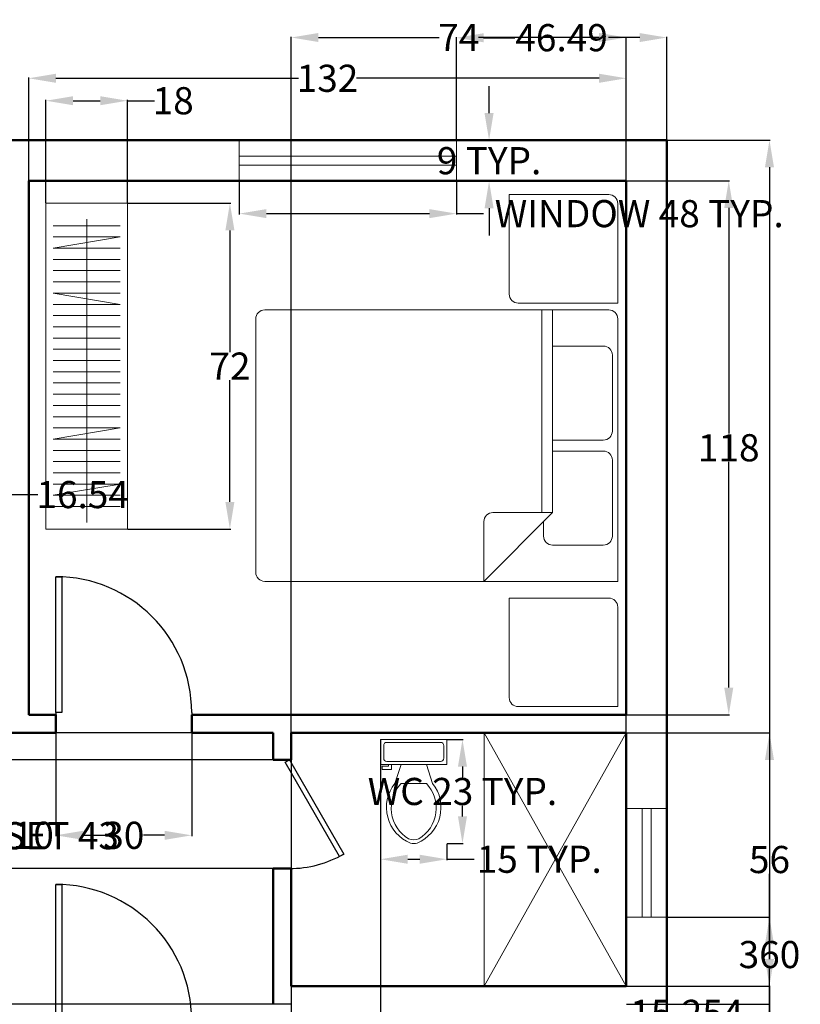
# Model space of a CAD drawing. Units: inches. Extents: x -8 to 300, y -428 to 46.
# Tile 4 of 4: x 122 to 294, y -172 to 46. Entities that reach past the tile are written whole.
import ezdxf

# ---------------------------------------------------------------- set-up
doc = ezdxf.new("R2010")
doc.units = ezdxf.units.IN
doc.header["$MEASUREMENT"] = 0
for name, color, linetype, lineweight in [('A-ANNO-DIMS', 2, 'Continuous', 18), ('A-DOOR', 3, 'Continuous', 25), ('A-FLOR-CASE', 9, 'Continuous', 18), ('A-FLOR-FIXT', 9, 'Continuous', 18), ('A-FURN', 8, 'Continuous', 18), ('A-GLAZ', 4, 'Continuous', 18), ('A-WALL', 7, 'Continuous', 50)]:
    doc.layers.add(name, color=color, linetype=linetype, lineweight=lineweight)
doc.styles.get("Standard").update_dxf_attribs({"font": 'arial.ttf'})
doc.dimstyles.get("Standard").update_dxf_attribs({"dimtxt": 6, "dimasz": 6, "dimexe": 0.18, "dimexo": 0.0625, "dimgap": 0.09, "dimtad": 0, "dimtih": 1, "dimtoh": 1, "dimdec": 0, "dimzin": 0, "dimdsep": 46, "dimlunit": 4, "dimtxsty": 'Standard', "dimcen": 0.09, "dimadec": 0, "dimazin": 0, "dimtfac": 1, "dimtdec": 0, "dimtofl": 0, "dimtmove": 0, "dimatfit": 3, "dimfxl": 1, "dimtolj": 1, "dimtzin": 0, "dimarcsym": 0})

# ---------------------------------------------------------------- blocks, each defined once
blk = doc.blocks.new('*U2')
for p, q in [((0, 0), (0, -6)), ((40, 0), (40, -6))]:
    blk.add_line(p, q)
blk.add_lwpolyline([(0, 0), (0, 40), (1.75, 40), (1.75, 0)], close=True)
blk.add_arc((0, 0), 40, 0, 90)
blk = doc.blocks.new('*U11')
for p, q in [((0, 0), (0, -6)), ((40, 0), (40, -6))]:
    blk.add_line(p, q)
blk.add_lwpolyline([(0, 0), (34.64, 20), (35.52, 18.48), (0.87, -1.52)], close=True)
blk.add_arc((0, 0), 40, 0, 30)
blk = doc.blocks.new('Toilet - top')
for p, q in [((9.5, -6), (9.5, -2)), ((-10, -8.5), (-8, -8.5)), ((-10, -9.5), (-10, -8.5)), ((-8, -8.5), (-8, -8)), ((-7, -8), (-7, -9.5)), ((-4, -8), (-6, -14)), ((4, -8), (6, -14)), ((-7, -9.5), (-10, -9.5)), ((4, -14), (-4, -14))]:
    blk.add_line(p, q)
blk.add_lwpolyline([(10.5, -8), (10.5, 0), (-10.5, 0), (-10.5, -8)], close=True)
for points in [[(-9.5, -2), (-9.5, -6)], [(8.5, -1), (-8.5, -1)], [(-8.5, -7), (8.5, -7)]]:
    blk.add_lwpolyline(points)
for centre, radius, start, end in [((-8.62, -1.88), 0.884, 81.8699, 188.1301), ((8.62, -1.88), 0.884, 351.8699, 98.1301), ((-8.62, -6.12), 0.884, 171.8699, 278.1301), ((8.62, -6.12), 0.884, 261.8699, 8.1301), ((3.52, -21.58), 12.17, 141.4691, 247.9714), ((4.2, -21.82), 11.33, 136.3677, 238.9468), ((-3.52, -21.58), 12.17, 292.0284, 38.5307), ((-4.2, -21.82), 11.33, 301.053, 43.6321), ((0, -27.88), 4, 245.7318, 294.2682), ((0, -29), 4, 254.8605, 285.1395)]:
    blk.add_arc(centre, radius, start, end)
blk = doc.blocks.new('Bed - Queen')
for p, q in [((2, 0), (60, 0)), ((60, 0), (60, -78)), ((0, -78), (0, -2)), ((10, -1.2), (26.8, -1.2)), ((33.2, -1.2), (50, -1.2)), ((8, -14.4), (8, -3.2)), ((28.8, -3.2), (28.8, -14.4)), ((31.2, -14.4), (31.2, -3.2)), ((52, -3.2), (52, -14.4)), ((0, -14.4), (44.8, -14.4)), ((60, -29.6), (44.8, -14.4)), ((44.8, -14.4), (44.8, -27.6)), ((44.8, -16.8), (0, -16.8)), ((50, -16.4), (46.8, -16.4)), ((46.8, -29.6), (60, -29.6)), ((58, -80), (2, -80))]:
    blk.add_line(p, q)
for points in [[(-1.48, 0), (-23.48, 0, 0.414214), (-25.48, -2), (-25.48, -24), (-3.48, -24, 0.414214), (-1.48, -22)], [(65.69, 0), (87.69, 0), (87.69, -22, -0.414214), (85.69, -24), (63.69, -24), (63.69, -2, -0.414214)]]:
    blk.add_lwpolyline(points, format="xyb", close=True)
for centre, start, end in [((2, -2), 90, 180), ((10, -3.2), 90, 180), ((26.8, -3.2), 0, 90), ((33.2, -3.2), 90, 180), ((50, -3.2), 0, 90), ((50, -14.4), 270, 0), ((46.8, -27.6), 180, 270), ((2, -78), 180, 270), ((58, -78), 270, 0)]:
    blk.add_arc(centre, 2, start, end)
blk = doc.blocks.new('WIN-48IN')
for p, q in [((0, 0), (0, 9)), ((48, 9), (48, 0)), ((0, 5.5), (48, 5.5)), ((0, 3.5), (48, 3.5))]:
    blk.add_line(p, q)
blk = doc.blocks.new('WIN-24IN')
for p, q in [((0, 24), (9, 24)), ((3.5, 24), (3.5, 0)), ((5.5, 24), (5.5, 0)), ((9, 0), (0, 0))]:
    blk.add_line(p, q)
blk = doc.blocks.new('*D15')
at = {"layer": 'A-ANNO-DIMS', "color": 0, "lineweight": -2, "transparency": 16777216}
for p, q in [((216.31, -113.16), (219.88, -113.16)), ((219.7, -119.16), (219.7, -121.48)), ((219.7, -130.19), (219.7, -127.87)), ((216.31, -136.19), (219.88, -136.19))]:
    blk.add_line(p, q, dxfattribs=at)
at = {"layer": 'A-ANNO-DIMS', "color": 0, "transparency": 16777216}
for points in [[(218.7, -119.16), (220.7, -119.16), (219.7, -113.16)], [(218.7, -130.19), (220.7, -130.19), (219.7, -136.19)]]:
    blk.add_solid(points, dxfattribs=at)
at = {"layer": 'Defpoints', "color": 0, "transparency": 16777216}
for p in [(216.25, -113.16), (219.7, -113.16), (216.25, -136.19)]:
    blk.add_point(p, dxfattribs=at)
at = {"layer": 'A-ANNO-DIMS', "color": 0, "transparency": 16777216, "insert": (219.7, -124.67), "char_height": 6, "attachment_point": 5}
blk.add_mtext('\\A1;WC 23 TYP.', dxfattribs=at)
blk = doc.blocks.new('*D16')
at = {"layer": 'A-ANNO-DIMS', "color": 0, "lineweight": -2, "transparency": 16777216}
for p, q in [((201.61, -136.25), (201.61, -139.83)), ((216.25, -136.25), (216.25, -139.83)), ((207.61, -139.65), (210.25, -139.65)), ((216.25, -139.65), (222.25, -139.65))]:
    blk.add_line(p, q, dxfattribs=at)
at = {"layer": 'A-ANNO-DIMS', "color": 0, "transparency": 16777216}
for points in [[(207.61, -138.65), (207.61, -140.65), (201.61, -139.65)], [(210.25, -138.65), (210.25, -140.65), (216.25, -139.65)]]:
    blk.add_solid(points, dxfattribs=at)
at = {"layer": 'Defpoints', "color": 0, "transparency": 16777216}
for p in [(201.61, -136.19), (216.25, -136.19), (216.25, -139.65)]:
    blk.add_point(p, dxfattribs=at)
at = {"layer": 'A-ANNO-DIMS', "color": 0, "transparency": 16777216, "insert": (236.66, -139.65), "char_height": 6, "attachment_point": 5}
blk.add_mtext('\\A1;15 TYP.', dxfattribs=at)
blk = doc.blocks.new('*D19')
at = {"layer": 'A-ANNO-DIMS', "color": 0, "lineweight": -2, "transparency": 16777216}
for p, q in [((170.38, 10.17), (170.38, 2.85)), ((218.38, 10.17), (218.38, 2.85)), ((176.38, 3.03), (212.38, 3.03)), ((218.38, 3.03), (224.38, 3.03))]:
    blk.add_line(p, q, dxfattribs=at)
at = {"layer": 'A-ANNO-DIMS', "color": 0, "transparency": 16777216}
for points in [[(176.38, 4.03), (176.38, 2.03), (170.38, 3.03)], [(212.38, 4.03), (212.38, 2.03), (218.38, 3.03)]]:
    blk.add_solid(points, dxfattribs=at)
at = {"layer": 'Defpoints', "color": 0, "transparency": 16777216}
for p in [(170.38, 10.23), (218.38, 10.23), (218.38, 3.03)]:
    blk.add_point(p, dxfattribs=at)
at = {"layer": 'A-ANNO-DIMS', "color": 0, "transparency": 16777216, "insert": (258.75, 3.03), "char_height": 6, "attachment_point": 5}
blk.add_mtext('\\A1;WINDOW 48 TYP.', dxfattribs=at)
blk = doc.blocks.new('*D20')
at = {"layer": 'A-ANNO-DIMS', "color": 0, "lineweight": -2, "transparency": 16777216}
for p, q in [((225.58, 25.23), (225.58, 31.23)), ((218.45, 19.23), (225.76, 19.23)), ((218.45, 10.23), (225.76, 10.23)), ((225.58, 4.23), (225.58, -1.77))]:
    blk.add_line(p, q, dxfattribs=at)
at = {"layer": 'A-ANNO-DIMS', "color": 0, "transparency": 16777216}
for points in [[(224.58, 25.23), (226.58, 25.23), (225.58, 19.23)], [(224.58, 4.23), (226.58, 4.23), (225.58, 10.23)]]:
    blk.add_solid(points, dxfattribs=at)
at = {"layer": 'Defpoints', "color": 0, "transparency": 16777216}
for p in [(218.38, 19.23), (225.58, 19.23), (218.38, 10.23)]:
    blk.add_point(p, dxfattribs=at)
at = {"layer": 'A-ANNO-DIMS', "color": 0, "transparency": 16777216, "insert": (225.58, 14.73), "char_height": 6, "attachment_point": 5}
blk.add_mtext('\\A1;9 TYP.', dxfattribs=at)
blk = doc.blocks.new('*D23')
at = {"layer": 'A-ANNO-DIMS', "color": 0, "lineweight": -2, "transparency": 16777216}
for p, q in [((37.97, -128.08), (37.97, -134.62)), ((80.78, -128.08), (80.78, -134.62)), ((43.97, -134.44), (74.78, -134.44)), ((80.78, -134.44), (86.78, -134.44))]:
    blk.add_line(p, q, dxfattribs=at)
at = {"layer": 'A-ANNO-DIMS', "color": 0, "transparency": 16777216}
for points in [[(43.97, -133.44), (43.97, -135.44), (37.97, -134.44)], [(74.78, -133.44), (74.78, -135.44), (80.78, -134.44)]]:
    blk.add_solid(points, dxfattribs=at)
at = {"layer": 'Defpoints', "color": 0, "transparency": 16777216}
for p in [(37.97, -128.02), (80.78, -128.02), (80.78, -134.44)]:
    blk.add_point(p, dxfattribs=at)
at = {"layer": 'A-ANNO-DIMS', "color": 0, "transparency": 16777216, "insert": (116.16, -134.44), "char_height": 6, "attachment_point": 5}
blk.add_mtext('\\A1;DINING SET 43', dxfattribs=at)
blk = doc.blocks.new('*D33')
at = {"layer": 'A-ANNO-DIMS', "color": 0, "lineweight": -2, "transparency": 16777216}
for p, q in [((264.94, 19.29), (287.71, 19.29)), ((287.53, 13.29), (287.53, -157.55)), ((287.53, -334.71), (287.53, -163.86)), ((264.94, -340.71), (287.71, -340.71))]:
    blk.add_line(p, q, dxfattribs=at)
at = {"layer": 'A-ANNO-DIMS', "color": 0, "transparency": 16777216}
for points in [[(286.53, 13.29), (288.53, 13.29), (287.53, 19.29)], [(286.53, -334.71), (288.53, -334.71), (287.53, -340.71)]]:
    blk.add_solid(points, dxfattribs=at)
at = {"layer": 'Defpoints', "color": 0, "transparency": 16777216}
for p in [(264.88, 19.29), (264.88, -340.71), (287.53, -340.71)]:
    blk.add_point(p, dxfattribs=at)
at = {"layer": 'A-ANNO-DIMS', "color": 0, "transparency": 16777216, "insert": (287.53, -160.71), "char_height": 6, "attachment_point": 5}
blk.add_mtext('\\A1;360', dxfattribs=at)
blk = doc.blocks.new('*D37')
at = {"layer": 'A-ANNO-DIMS', "color": 0, "lineweight": -2, "transparency": 16777216}
for p, q in [((123.88, 10.36), (123.88, 33.12)), ((129.88, 32.94), (183.47, 32.94)), ((249.88, 32.94), (196.28, 32.94)), ((255.88, 10.36), (255.88, 33.12))]:
    blk.add_line(p, q, dxfattribs=at)
at = {"layer": 'A-ANNO-DIMS', "color": 0, "transparency": 16777216}
for points in [[(129.88, 33.94), (129.88, 31.94), (123.88, 32.94)], [(249.88, 33.94), (249.88, 31.94), (255.88, 32.94)]]:
    blk.add_solid(points, dxfattribs=at)
at = {"layer": 'Defpoints', "color": 0, "transparency": 16777216}
for p in [(255.88, 32.94), (123.88, 10.29), (255.88, 10.29)]:
    blk.add_point(p, dxfattribs=at)
at = {"layer": 'A-ANNO-DIMS', "color": 0, "transparency": 16777216, "insert": (189.88, 32.94), "char_height": 6, "attachment_point": 5}
blk.add_mtext('\\A1;132', dxfattribs=at)
blk = doc.blocks.new('*D39')
at = {"layer": 'A-ANNO-DIMS', "color": 0, "lineweight": -2, "transparency": 16777216}
for p, q in [((255.94, 10.29), (278.71, 10.29)), ((278.53, 4.29), (278.53, -45.55)), ((278.53, -101.71), (278.53, -51.86)), ((255.94, -107.71), (278.71, -107.71))]:
    blk.add_line(p, q, dxfattribs=at)
at = {"layer": 'A-ANNO-DIMS', "color": 0, "transparency": 16777216}
for points in [[(277.53, 4.29), (279.53, 4.29), (278.53, 10.29)], [(277.53, -101.71), (279.53, -101.71), (278.53, -107.71)]]:
    blk.add_solid(points, dxfattribs=at)
at = {"layer": 'Defpoints', "color": 0, "transparency": 16777216}
for p in [(255.88, 10.29), (255.88, -107.71), (278.53, -107.71)]:
    blk.add_point(p, dxfattribs=at)
at = {"layer": 'A-ANNO-DIMS', "color": 0, "transparency": 16777216, "insert": (278.53, -48.71), "char_height": 6, "attachment_point": 5}
blk.add_mtext('\\A1;118', dxfattribs=at)
blk = doc.blocks.new('*D44')
at = {"layer": 'A-ANNO-DIMS', "color": 0, "lineweight": -2, "transparency": 16777216}
for p, q in [((129.88, -111.77), (129.88, -134.54)), ((159.88, -111.77), (159.88, -134.54)), ((135.88, -134.36), (140.5, -134.36)), ((153.88, -134.36), (149.25, -134.36))]:
    blk.add_line(p, q, dxfattribs=at)
at = {"layer": 'A-ANNO-DIMS', "color": 0, "transparency": 16777216}
for points in [[(135.88, -133.36), (135.88, -135.36), (129.88, -134.36)], [(153.88, -133.36), (153.88, -135.36), (159.88, -134.36)]]:
    blk.add_solid(points, dxfattribs=at)
at = {"layer": 'Defpoints', "color": 0, "transparency": 16777216}
for p in [(129.88, -111.71), (159.88, -111.71), (129.88, -134.36)]:
    blk.add_point(p, dxfattribs=at)
at = {"layer": 'A-ANNO-DIMS', "color": 0, "transparency": 16777216, "insert": (144.88, -134.36), "char_height": 6, "attachment_point": 5}
blk.add_mtext('\\A1;30', dxfattribs=at)
blk = doc.blocks.new('*D45')
at = {"layer": 'A-ANNO-DIMS', "color": 0, "lineweight": -2, "transparency": 16777216}
for p, q in [((119.875934, -111.769234), (119.875934, -134.536734)), ((129.875934, -111.769234), (129.875934, -134.536734)), ((113.875934, -134.356734), (107.875934, -134.356734)), ((135.875934, -134.356734), (141.875934, -134.356734))]:
    blk.add_line(p, q, dxfattribs=at)
at = {"layer": 'A-ANNO-DIMS', "color": 0, "transparency": 16777216}
for points in [[(113.875934, -133.356734), (113.875934, -135.356734), (119.875934, -134.356734)], [(135.875934, -133.356734), (135.875934, -135.356734), (129.875934, -134.356734)]]:
    blk.add_solid(points, dxfattribs=at)
at = {"layer": 'Defpoints', "color": 0, "transparency": 16777216}
for p in [(119.875934, -111.706734), (129.875934, -111.706734), (119.875934, -134.356734)]:
    blk.add_point(p, dxfattribs=at)
at = {"layer": 'A-ANNO-DIMS', "color": 0, "transparency": 16777216, "insert": (124.875934, -134.356734), "char_height": 6, "attachment_point": 5}
blk.add_mtext('\\A1;10', dxfattribs=at)
blk = doc.blocks.new('*D47')
at = {"layer": 'A-ANNO-DIMS', "color": 0, "lineweight": -2, "transparency": 16777216}
for p, q in [((103.33, -81.64), (103.33, -58.88)), ((109.33, -59.06), (113.88, -59.06)), ((119.88, -81.64), (119.88, -58.88)), ((119.88, -59.06), (125.88, -59.06))]:
    blk.add_line(p, q, dxfattribs=at)
at = {"layer": 'A-ANNO-DIMS', "color": 0, "transparency": 16777216}
for points in [[(109.33, -58.06), (109.33, -60.06), (103.33, -59.06)], [(113.88, -58.06), (113.88, -60.06), (119.88, -59.06)]]:
    blk.add_solid(points, dxfattribs=at)
at = {"layer": 'Defpoints', "color": 0, "transparency": 16777216}
for p in [(119.88, -59.06), (103.33, -81.71), (119.88, -81.71)]:
    blk.add_point(p, dxfattribs=at)
at = {"layer": 'A-ANNO-DIMS', "color": 0, "transparency": 16777216, "insert": (135.79, -59.06), "char_height": 6, "attachment_point": 5}
blk.add_mtext('\\A1;16.54', dxfattribs=at)
blk = doc.blocks.new('*D49')
at = {"layer": 'A-ANNO-DIMS', "color": 0, "lineweight": -2, "transparency": 16777216}
for p, q in [((218.38, 19.29), (218.35, 42.06)), ((224.35, 41.89), (231.26, 41.9)), ((258.85, 41.94), (251.94, 41.93)), ((264.88, 19.36), (264.85, 42.12))]:
    blk.add_line(p, q, dxfattribs=at)
at = {"layer": 'A-ANNO-DIMS', "color": 0, "transparency": 16777216}
for points in [[(224.35, 42.89), (224.36, 40.89), (218.35, 41.88)], [(258.84, 42.94), (258.85, 40.94), (264.85, 41.94)]]:
    blk.add_solid(points, dxfattribs=at)
at = {"layer": 'Defpoints', "color": 0, "transparency": 16777216}
for p in [(264.85, 41.94), (218.38, 19.23), (264.88, 19.29)]:
    blk.add_point(p, dxfattribs=at)
at = {"layer": 'A-ANNO-DIMS', "color": 0, "transparency": 16777216, "insert": (241.6, 41.91), "char_height": 6, "attachment_point": 5}
blk.add_mtext('\\A1;46.49', dxfattribs=at)
blk = doc.blocks.new('*D52')
at = {"layer": 'A-ANNO-DIMS', "color": 0, "lineweight": -2, "transparency": 16777216}
for p, q in [((181.88, -111.64), (181.88, 42.13)), ((187.88, 41.95), (214.53, 41.95)), ((249.88, 41.95), (223.23, 41.95)), ((255.88, -111.64), (255.88, 42.13))]:
    blk.add_line(p, q, dxfattribs=at)
at = {"layer": 'A-ANNO-DIMS', "color": 0, "transparency": 16777216}
for points in [[(187.88, 42.95), (187.88, 40.95), (181.88, 41.95)], [(249.88, 42.95), (249.88, 40.95), (255.88, 41.95)]]:
    blk.add_solid(points, dxfattribs=at)
at = {"layer": 'Defpoints', "color": 0, "transparency": 16777216}
for p in [(255.88, 41.95), (181.88, -111.71), (255.88, -111.71)]:
    blk.add_point(p, dxfattribs=at)
at = {"layer": 'A-ANNO-DIMS', "color": 0, "transparency": 16777216, "insert": (218.88, 41.95), "char_height": 6, "attachment_point": 5}
blk.add_mtext('\\A1;74', dxfattribs=at)
blk = doc.blocks.new('*D53')
at = {"layer": 'A-ANNO-DIMS', "color": 0, "lineweight": -2, "transparency": 16777216}
for p, q in [((255.94, -111.71), (287.71, -111.71)), ((287.53, -117.71), (287.53, -136.55)), ((287.53, -161.71), (287.53, -142.86)), ((255.94, -167.71), (287.71, -167.71))]:
    blk.add_line(p, q, dxfattribs=at)
at = {"layer": 'A-ANNO-DIMS', "color": 0, "transparency": 16777216}
for points in [[(286.53, -117.71), (288.53, -117.71), (287.53, -111.71)], [(286.53, -161.71), (288.53, -161.71), (287.53, -167.71)]]:
    blk.add_solid(points, dxfattribs=at)
at = {"layer": 'Defpoints', "color": 0, "transparency": 16777216}
for p in [(255.88, -111.71), (255.88, -167.71), (287.53, -167.71)]:
    blk.add_point(p, dxfattribs=at)
at = {"layer": 'A-ANNO-DIMS', "color": 0, "transparency": 16777216, "insert": (287.53, -139.71), "char_height": 6, "attachment_point": 5}
blk.add_mtext('\\A1;56', dxfattribs=at)
blk = doc.blocks.new('*D55')
at = {"layer": 'A-ANNO-DIMS', "color": 0, "lineweight": -2, "transparency": 16777216}
for p, q in [((287.53, -161.71), (287.53, -155.71)), ((255.94, -167.71), (287.71, -167.71)), ((255.94, -171.71), (287.71, -171.71)), ((287.53, -177.71), (287.53, -183.71)), ((287.53, -183.71), (281.53, -183.71))]:
    blk.add_line(p, q, dxfattribs=at)
at = {"layer": 'A-ANNO-DIMS', "color": 0, "transparency": 16777216}
for points in [[(286.53, -161.71), (288.53, -161.71), (287.53, -167.71)], [(286.53, -177.71), (288.53, -177.71), (287.53, -171.71)]]:
    blk.add_solid(points, dxfattribs=at)
at = {"layer": 'Defpoints', "color": 0, "transparency": 16777216}
for p in [(255.88, -167.71), (255.88, -171.71), (287.53, -171.71)]:
    blk.add_point(p, dxfattribs=at)
at = {"layer": 'A-ANNO-DIMS', "color": 0, "transparency": 16777216, "insert": (279.36, -183.71), "char_height": 6, "attachment_point": 5}
blk.add_mtext('\\A1;4', dxfattribs=at)
blk = doc.blocks.new('*D56')
at = {"layer": 'A-ANNO-DIMS', "color": 0, "lineweight": -2, "transparency": 16777216}
for p, q in [((177.81, -117.71), (2.05, -117.71)), ((2.23, -123.71), (2.23, -126.6)), ((2.23, -135.71), (2.23, -132.81)), ((177.81, -141.71), (2.05, -141.71))]:
    blk.add_line(p, q, dxfattribs=at)
at = {"layer": 'A-ANNO-DIMS', "color": 0, "transparency": 16777216}
for points in [[(1.23, -123.71), (3.23, -123.71), (2.23, -117.71)], [(1.23, -135.71), (3.23, -135.71), (2.23, -141.71)]]:
    blk.add_solid(points, dxfattribs=at)
at = {"layer": 'Defpoints', "color": 0, "transparency": 16777216}
for p in [(177.88, -117.71), (2.23, -141.71), (177.88, -141.71)]:
    blk.add_point(p, dxfattribs=at)
at = {"layer": 'A-ANNO-DIMS', "color": 0, "transparency": 16777216, "insert": (2.23, -129.71), "char_height": 6, "attachment_point": 5}
blk.add_mtext('\\A1;24', dxfattribs=at)
blk = doc.blocks.new('*D57')
at = {"layer": 'A-ANNO-DIMS', "color": 0, "lineweight": -2, "transparency": 16777216}
for p, q in [((2.23, -105.71), (2.23, -99.71)), ((177.81, -111.71), (2.05, -111.71)), ((177.81, -117.71), (2.05, -117.71)), ((2.23, -123.71), (2.23, -129.71)), ((2.23, -129.71), (-3.77, -129.71))]:
    blk.add_line(p, q, dxfattribs=at)
at = {"layer": 'A-ANNO-DIMS', "color": 0, "transparency": 16777216}
for points in [[(1.23, -105.71), (3.23, -105.71), (2.23, -111.71)], [(1.23, -123.71), (3.23, -123.71), (2.23, -117.71)]]:
    blk.add_solid(points, dxfattribs=at)
at = {"layer": 'Defpoints', "color": 0, "transparency": 16777216}
for p in [(177.88, -111.71), (2.23, -117.71), (177.88, -117.71)]:
    blk.add_point(p, dxfattribs=at)
at = {"layer": 'A-ANNO-DIMS', "color": 0, "transparency": 16777216, "insert": (-5.84, -129.71), "char_height": 6, "attachment_point": 5}
blk.add_mtext('\\A1;6', dxfattribs=at)
blk = doc.blocks.new('*D58')
at = {"layer": 'A-ANNO-DIMS', "color": 0, "lineweight": -2, "transparency": 16777216}
for p, q in [((2.225934, -165.706734), (2.225934, -159.706734)), ((181.813434, -171.706734), (2.045934, -171.706734)), ((177.813434, -179.706734), (2.045934, -179.706734)), ((2.225934, -185.706734), (2.225934, -191.706734))]:
    blk.add_line(p, q, dxfattribs=at)
at = {"layer": 'A-ANNO-DIMS', "color": 0, "transparency": 16777216}
for points in [[(1.225934, -165.706734), (3.225934, -165.706734), (2.225934, -171.706734)], [(1.225934, -185.706734), (3.225934, -185.706734), (2.225934, -179.706734)]]:
    blk.add_solid(points, dxfattribs=at)
at = {"layer": 'Defpoints', "color": 0, "transparency": 16777216}
for p in [(2.225934, -171.706734), (181.875934, -171.706734), (177.875934, -179.706734)]:
    blk.add_point(p, dxfattribs=at)
at = {"layer": 'A-ANNO-DIMS', "color": 0, "transparency": 16777216, "insert": (2.225934, -175.706734), "char_height": 6, "attachment_point": 5}
blk.add_mtext('\\A1;8', dxfattribs=at)
blk = doc.blocks.new('*D61')
at = {"layer": 'A-ANNO-DIMS', "color": 0, "lineweight": -2, "transparency": 16777216}
for p, q in [((264.94, -152.45), (287.71, -152.45)), ((287.53, -158.45), (287.53, -161.71)), ((255.94, -167.71), (287.71, -167.71)), ((287.53, -167.71), (287.53, -173.71)), ((287.53, -173.71), (281.53, -173.71))]:
    blk.add_line(p, q, dxfattribs=at)
at = {"layer": 'A-ANNO-DIMS', "color": 0, "transparency": 16777216}
for points in [[(286.53, -158.45), (288.53, -158.45), (287.53, -152.45)], [(286.53, -161.71), (288.53, -161.71), (287.53, -167.71)]]:
    blk.add_solid(points, dxfattribs=at)
at = {"layer": 'Defpoints', "color": 0, "transparency": 16777216}
for p in [(264.88, -152.45), (255.88, -167.71), (287.53, -167.71)]:
    blk.add_point(p, dxfattribs=at)
at = {"layer": 'A-ANNO-DIMS', "color": 0, "transparency": 16777216, "insert": (269.28, -173.71), "char_height": 6, "attachment_point": 5}
blk.add_mtext('\\A1;15.254', dxfattribs=at)
blk = doc.blocks.new('*D63')
at = {"layer": 'A-ANNO-DIMS', "color": 0, "lineweight": -2, "transparency": 16777216}
for p, q in [((181.88, -111.77), (181.88, -424.4)), ((201.61, -113.22), (201.61, -424.4)), ((187.88, -424.22), (195.61, -424.22)), ((201.61, -424.22), (207.61, -424.22))]:
    blk.add_line(p, q, dxfattribs=at)
at = {"layer": 'A-ANNO-DIMS', "color": 0, "transparency": 16777216}
for points in [[(187.88, -423.22), (187.88, -425.22), (181.88, -424.22)], [(195.61, -423.22), (195.61, -425.22), (201.61, -424.22)]]:
    blk.add_solid(points, dxfattribs=at)
at = {"layer": 'Defpoints', "color": 0, "transparency": 16777216}
for p in [(181.88, -111.71), (201.61, -113.16), (201.61, -424.22)]:
    blk.add_point(p, dxfattribs=at)
at = {"layer": 'A-ANNO-DIMS', "color": 0, "transparency": 16777216, "insert": (219.86, -424.22), "char_height": 6, "attachment_point": 5}
blk.add_mtext('\\A1;19.734', dxfattribs=at)
blk = doc.blocks.new('*D67')
at = {"layer": 'A-ANNO-DIMS', "color": 0, "lineweight": -2, "transparency": 16777216}
for p, q in [((127.67, 5.39), (127.67, 28.16)), ((133.67, 27.98), (139.67, 27.98)), ((145.67, 5.39), (145.67, 28.16)), ((145.67, 27.98), (151.67, 27.98))]:
    blk.add_line(p, q, dxfattribs=at)
at = {"layer": 'A-ANNO-DIMS', "color": 0, "transparency": 16777216}
for points in [[(133.67, 28.98), (133.67, 26.98), (127.67, 27.98)], [(139.67, 28.98), (139.67, 26.98), (145.67, 27.98)]]:
    blk.add_solid(points, dxfattribs=at)
at = {"layer": 'Defpoints', "color": 0, "transparency": 16777216}
for p in [(145.67, 27.98), (127.67, 5.33), (145.67, 5.33)]:
    blk.add_point(p, dxfattribs=at)
at = {"layer": 'A-ANNO-DIMS', "color": 0, "transparency": 16777216, "insert": (155.79, 27.98), "char_height": 6, "attachment_point": 5}
blk.add_mtext('\\A1;18', dxfattribs=at)
blk = doc.blocks.new('*D68')
at = {"layer": 'A-ANNO-DIMS', "color": 0, "lineweight": -2, "transparency": 16777216}
for p, q in [((145.74, 5.33), (168.5, 5.33)), ((168.32, -0.67), (168.32, -27.57)), ((168.32, -60.67), (168.32, -33.77)), ((145.74, -66.67), (168.5, -66.67))]:
    blk.add_line(p, q, dxfattribs=at)
at = {"layer": 'A-ANNO-DIMS', "color": 0, "transparency": 16777216}
for points in [[(167.32, -0.67), (169.32, -0.67), (168.32, 5.33)], [(167.32, -60.67), (169.32, -60.67), (168.32, -66.67)]]:
    blk.add_solid(points, dxfattribs=at)
at = {"layer": 'Defpoints', "color": 0, "transparency": 16777216}
for p in [(145.67, 5.33), (145.67, -66.67), (168.32, -66.67)]:
    blk.add_point(p, dxfattribs=at)
at = {"layer": 'A-ANNO-DIMS', "color": 0, "transparency": 16777216, "insert": (168.32, -30.67), "char_height": 6, "attachment_point": 5}
blk.add_mtext('\\A1;72', dxfattribs=at)

msp = doc.modelspace()

# ---------------------------------------------------------------- linework, layer by layer
at = {"layer": 'A-FLOR-CASE'}
for p, q in [((144.1061, 0.3622), (129.2823, 0.3622)), ((136.6746, 1.8026), (136.6746, -65.2319)), ((144.1061, -2.1205), (129.2823, -2.1205)), ((144.1061, -2.1205), (129.2823, -4.6033)), ((144.1061, -4.6033), (129.2823, -4.6033)), ((144.1061, -7.086), (129.2823, -7.086)), ((144.1061, -9.5688), (129.2823, -9.5688)), ((144.1061, -12.0516), (129.2823, -12.0516)), ((144.1061, -14.5343), (129.2823, -14.5343)), ((129.2823, -14.5343), (144.1061, -17.0171)), ((144.1061, -17.0171), (129.2823, -17.0171)), ((144.1061, -19.4998), (129.2823, -19.4998)), ((144.1061, -21.9826), (129.2823, -21.9826)), ((144.1061, -24.4654), (129.2823, -24.4654)), ((144.1061, -26.9481), (129.2823, -26.9481)), ((144.1061, -29.4309), (129.2823, -29.4309)), ((144.1061, -31.9136), (129.2823, -31.9136)), ((144.1061, -34.3964), (129.2823, -34.3964)), ((144.1061, -36.8791), (129.2823, -36.8791)), ((144.1061, -39.3619), (129.2823, -39.3619)), ((144.1061, -41.8447), (129.2823, -41.8447)), ((144.1061, -44.3274), (129.2823, -44.3274)), ((144.1061, -44.3274), (129.2823, -46.8102)), ((144.1061, -46.8102), (129.2823, -46.8102)), ((144.1061, -49.2929), (129.2823, -49.2929)), ((144.1061, -51.7757), (129.2823, -51.7757)), ((144.1061, -54.2585), (129.2823, -54.2585)), ((144.1061, -56.7412), (129.2823, -56.7412)), ((144.1061, -56.7412), (129.2823, -59.224)), ((144.1061, -59.224), (129.2823, -59.224)), ((144.1061, -61.7067), (129.2823, -61.7067))]:
    msp.add_line(p, q, dxfattribs=at)
msp.add_lwpolyline([(127.6746, -66.6723), (127.6746, 5.3277), (145.6746, 5.3277), (145.6746, -66.6723), (127.6746, -66.6723), (145.6746, -66.6723)], dxfattribs=at)
at = {"layer": 'A-FLOR-FIXT'}
for p, q in [((224.4854, -111.7067), (255.8759, -167.7067)), ((255.8759, -111.7067), (224.4854, -167.7067))]:
    msp.add_line(p, q, dxfattribs=at)
msp.add_lwpolyline([(255.8759, -111.7067), (224.4854, -111.7067), (224.4854, -167.7067), (255.8759, -167.7067)], close=True, dxfattribs=at)
for points in [[(224.4854, -153.7067), (224.4854, -167.7067)], [(255.8759, -167.7067), (255.8759, -153.7067)]]:
    msp.add_lwpolyline(points, dxfattribs=at)
at = {"layer": 'A-WALL'}
for p, q in [((123.8759, 10.2933), (123.8759, -107.7067)), ((123.8759, 10.2933), (255.8759, 10.2933)), ((255.8759, 10.2933), (255.8759, -107.7067)), ((123.8759, -107.7067), (129.8759, -107.7067)), ((129.8759, -107.7067), (129.8759, -111.7067)), ((159.8759, -107.7067), (159.8759, -111.7067)), ((159.8759, -107.7067), (255.8759, -107.7067)), ((119.8759, -111.7067), (129.8759, -111.7067)), ((159.8759, -111.7067), (177.8759, -111.7067)), ((177.8759, -111.7067), (177.8759, -117.7067)), ((181.8759, -111.7067), (181.8759, -117.7067)), ((181.8759, -111.7067), (255.8759, -111.7067)), ((255.8759, -111.7067), (255.8759, -167.7067)), ((181.8759, -117.7067), (177.8759, -117.7067)), ((181.8759, -141.7067), (177.8759, -141.7067)), ((177.8759, -141.7067), (177.8759, -167.7067)), ((181.8759, -141.7067), (181.8759, -167.7067)), ((177.8759, -167.7067), (177.8759, -171.7067)), ((181.8759, -167.7067), (255.8759, -167.7067))]:
    msp.add_line(p, q, dxfattribs=at)
msp.add_lwpolyline([(39.8759, -340.7067), (24.8759, -340.7067), (24.8759, 19.2933), (264.8759, 19.2933), (264.8759, -340.7067), (197.0947, -340.7067)], dxfattribs=at)

# ---------------------------------------------------------------- block references
at = {"layer": 'A-DOOR', "xscale": 0.75, "yscale": 0.75, "zscale": 0.75}
for p in [(129.8759, -107.2067), (129.8759, -175.2067)]:
    msp.add_blockref('*U2', p, dxfattribs=at)
at = {"layer": 'A-DOOR', "xscale": 0.6, "yscale": 0.6, "zscale": 0.6, "rotation": 270}
msp.add_blockref('*U11', (181.4759, -117.7067), dxfattribs=at)
at = {"layer": 'A-FLOR-FIXT', "xscale": 0.6970645332664974, "yscale": 0.6970645332664974, "zscale": 0.6970645332664974}
msp.add_blockref('Toilet - top', (208.9291, -113.157), dxfattribs=at)
at = {"layer": 'A-FURN', "rotation": 270}
msp.add_blockref('Bed - Queen', (254.0205, -18.2368), dxfattribs=at)
at = {"layer": 'A-GLAZ'}
for name, p in [('WIN-48IN', (170.384, 10.231)), ('WIN-24IN', (255.876, -152.453))]:
    msp.add_blockref(name, p, dxfattribs=at)

# ---------------------------------------------------------------- dimensions: what is measured, and where the dimension line sits
at = {"layer": 'A-ANNO-DIMS'}
for base, p1, p2, override, picture, middle in [((255.8759, 41.9496), (181.8759, -111.7067), (255.8759, -111.7067), {"dimdec": 0, "dimlfac": 1, "dimrnd": 0, "dimzin": 0, "dimdsep": 46, "dimlunit": 2}, '*D52', (218.8759, 41.9496)), ((255.8759, 32.9433), (123.8759, 10.2933), (255.8759, 10.2933), {"dimdec": 0, "dimlfac": 1, "dimrnd": 0, "dimzin": 0, "dimdsep": 46, "dimlunit": 2}, '*D37', (189.8759, 32.9433)), ((145.6746, 27.9777), (127.6746, 5.3277), (145.6746, 5.3277), {"dimdec": 0, "dimlfac": 1, "dimrnd": 0, "dimzin": 0, "dimdsep": 46, "dimlunit": 2}, '*D67', (155.7857, 27.9777)), ((119.8759, -59.0567), (103.335, -81.7067), (119.8759, -81.7067), {"dimdec": 2, "dimlfac": 1, "dimrnd": 0, "dimzin": 0, "dimdsep": 46, "dimlunit": 2}, '*D47', (135.7947, -59.0567)), ((201.6099, -424.2177), (181.8759, -111.7067), (201.6099, -113.157), {"dimdec": 3, "dimlfac": 1, "dimrnd": 0, "dimzin": 0, "dimdsep": 46, "dimlunit": 2}, '*D63', (219.8595, -424.2177))]:
    dim = msp.add_linear_dim(base=base, p1=p1, p2=p2, dimstyle='Standard', override=override, dxfattribs=at)
    dim.commit()
    dim.dimension.update_dxf_attribs({"geometry": picture, "text_midpoint": middle})
for base, p1, p2, angle, override, picture, middle in [((264.8457, 41.9432), (218.3841, 19.2312), (264.8759, 19.2933), 0.076535, {"dimdec": 2, "dimlfac": 1, "dimrnd": 0, "dimzin": 0, "dimdsep": 46, "dimlunit": 2}, '*D49', (241.5998, 41.9122)), ((287.5259, -340.7067), (264.8759, 19.2933), (264.8759, -340.7067), 90, {"dimdec": 0, "dimlfac": 1, "dimrnd": 0, "dimzin": 0, "dimdsep": 46, "dimlunit": 2}, '*D33', (287.5259, -160.7067)), ((278.5259, -107.7067), (255.8759, 10.2933), (255.8759, -107.7067), 270, {"dimdec": 0, "dimlfac": 1, "dimrnd": 0, "dimzin": 0, "dimdsep": 46, "dimlunit": 2}, '*D39', (278.5259, -48.7067)), ((168.3246, -66.6723), (145.6746, 5.3277), (145.6746, -66.6723), 270, {"dimdec": 0, "dimlfac": 1, "dimrnd": 0, "dimzin": 0, "dimdsep": 46, "dimlunit": 2}, '*D68', (168.3246, -30.6723)), ((2.2259, -117.7067), (177.8759, -111.7067), (177.8759, -117.7067), 90, {"dimdec": 0, "dimlfac": 1, "dimrnd": 0, "dimzin": 0, "dimdsep": 46, "dimlunit": 2}, '*D57', (-5.845, -129.7067)), ((119.8759, -134.3567), (129.8759, -111.7067), (119.8759, -111.7067), 180, {"dimdec": 0, "dimlfac": 1, "dimrnd": 0, "dimzin": 0, "dimdsep": 46, "dimlunit": 2}, '*D45', (124.8759, -134.3567)), ((129.8759, -134.3567), (159.8759, -111.7067), (129.8759, -111.7067), 180, {"dimdec": 0, "dimlfac": 1, "dimrnd": 0, "dimzin": 0, "dimdsep": 46, "dimlunit": 2}, '*D44', (144.8759, -134.3567)), ((287.5259, -167.7067), (255.8759, -111.7067), (255.8759, -167.7067), 90, {"dimdec": 0, "dimlfac": 1, "dimrnd": 0, "dimzin": 0, "dimdsep": 46, "dimlunit": 2}, '*D53', (287.5259, -139.7067)), ((2.2259, -141.7067), (177.8759, -117.7067), (177.8759, -141.7067), 90, {"dimdec": 0, "dimlfac": 1, "dimrnd": 0, "dimzin": 0, "dimdsep": 46, "dimlunit": 2}, '*D56', (2.2259, -129.7067)), ((287.5259, -167.7067), (264.8759, -152.453), (255.8759, -167.7067), 90, {"dimdec": 3, "dimlfac": 1, "dimrnd": 0, "dimzin": 0, "dimdsep": 46, "dimlunit": 2}, '*D61', (269.2763, -173.7067)), ((287.5259, -171.7067), (255.8759, -167.7067), (255.8759, -171.7067), 90, {"dimdec": 0, "dimlfac": 1, "dimrnd": 0, "dimzin": 0, "dimdsep": 46, "dimlunit": 2}, '*D55', (279.3609, -183.7067)), ((2.2259, -171.7067), (177.8759, -179.7067), (181.8759, -171.7067), 90, {"dimdec": 0, "dimlfac": 1, "dimrnd": 0, "dimzin": 0, "dimdsep": 46, "dimlunit": 2}, '*D58', (2.2259, -175.7067))]:
    dim = msp.add_linear_dim(base=base, p1=p1, p2=p2, angle=angle, dimstyle='Standard', override=override, dxfattribs=at)
    dim.commit()
    dim.dimension.update_dxf_attribs({"geometry": picture, "text_midpoint": middle})
for base, p1, p2, text, picture, middle in [((225.5841, 19.2312), (218.3841, 10.2312), (218.3841, 19.2312), '<> TYP.', '*D20', (225.5841, 14.7312)), ((219.7036, -113.157), (216.2482, -136.1924), (216.2482, -113.157), 'WC <> TYP.', '*D15', (219.7036, -124.6747))]:
    dim = msp.add_linear_dim(base=base, p1=p1, p2=p2, angle=90, text=text, dimstyle='Standard', override={"dimdec": 0, "dimlfac": 1, "dimrnd": 0, "dimzin": 0, "dimdsep": 46, "dimlunit": 2}, dxfattribs=at)
    dim.commit()
    dim.dimension.update_dxf_attribs({"geometry": picture, "text_midpoint": middle})
for base, p1, p2, text, picture, middle in [((218.3841, 3.0312), (170.3841, 10.2312), (218.3841, 10.2312), 'WINDOW <> TYP.', '*D19', (258.7531, 3.0312)), ((80.7776, -134.4366), (37.9711, -128.0156), (80.7776, -128.0156), 'DINING SET <>', '*D23', (116.1637, -134.4366)), ((216.2482, -139.6477), (201.6099, -136.1924), (216.2482, -136.1924), '<> TYP.', '*D16', (236.6588, -139.6477))]:
    dim = msp.add_linear_dim(base=base, p1=p1, p2=p2, text=text, dimstyle='Standard', override={"dimdec": 0, "dimlfac": 1, "dimrnd": 0, "dimzin": 0, "dimdsep": 46, "dimlunit": 2}, dxfattribs=at)
    dim.commit()
    dim.dimension.update_dxf_attribs({"geometry": picture, "text_midpoint": middle})

doc.saveas('drawing.dxf')
